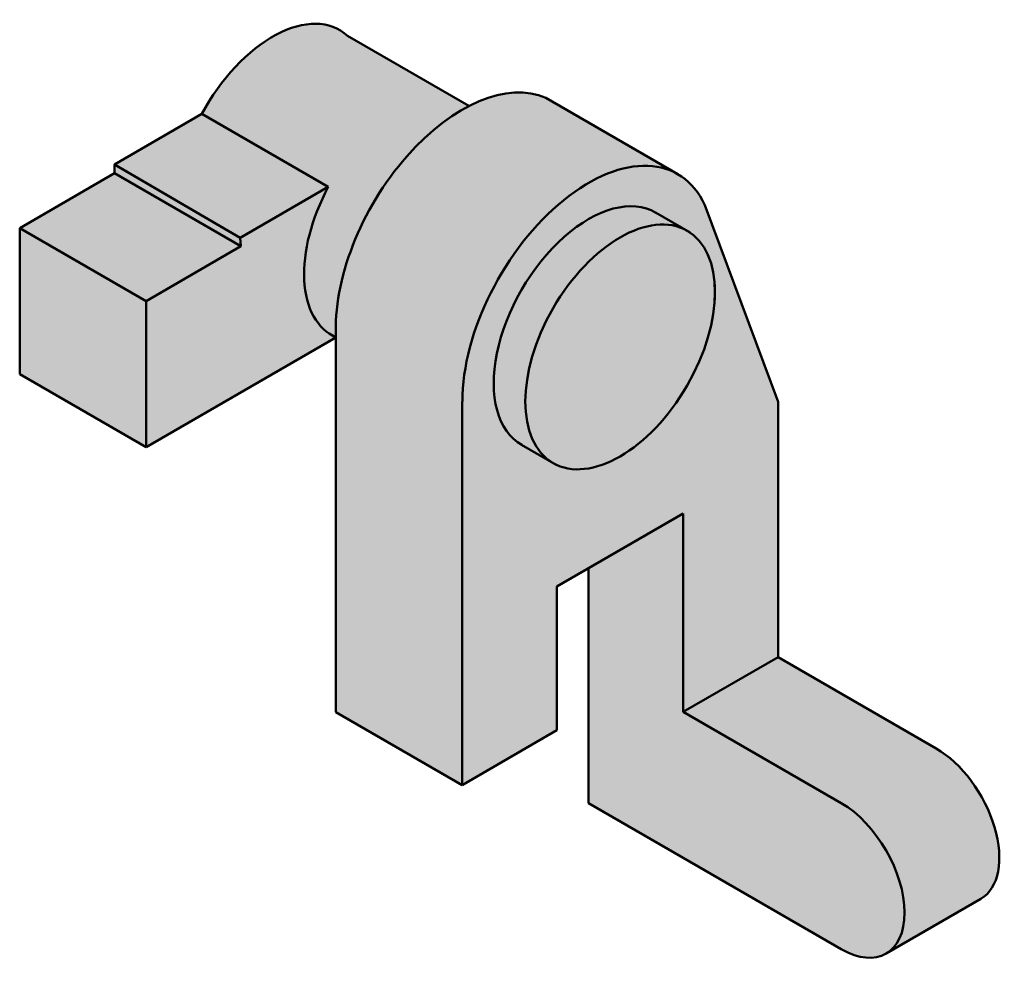
# Model space of a CAD drawing. Units: millimetres. Extents: x -330 to -195, y 135 to 265.
import ezdxf

# ---------------------------------------------------------------- set-up
doc = ezdxf.new("R2010")
doc.units = ezdxf.units.MM
doc.header["$MEASUREMENT"] = 0
doc.layers.add('M-HATC', color=18, linetype='Continuous', lineweight=18)
doc.layers.add('M-OUTL', color=18, linetype='Continuous', lineweight=50)

msp = doc.modelspace()

# ---------------------------------------------------------------- hatches: boundary and pattern name
at = {"layer": 'M-HATC'}
h = msp.add_hatch(color=256, dxfattribs=at)
h.dxf.hatch_style = 1
h.set_gradient(color1=(205, 105, 40), color2=(254, 234, 185), tint=1)
edge = h.paths.add_edge_path()
edge.add_line((-239.4440334627808, 243.7158516808131), (-257.507454304211, 254.1447725660983))
edge.add_ellipse((-268.9894374735072, 232.5417108040857), major_axis=(-12.24744871391589, -21.21320343559643), ratio=0.577350269189626, start_angle=182.0094469365693, end_angle=207.4091084575104)
edge.add_ellipse((-268.9894374735072, 232.5417108040857), major_axis=(-12.24744871391589, -21.21320343559643), ratio=0.577350269189626, start_angle=207.4091084575104, end_angle=332.9239439551128)
edge.add_line((-286.2780511034371, 221.3469536046194), (-286.2780511034371, 170.0048822703966))
edge.add_line((-286.2780511034371, 170.0048822703966), (-268.9894374735072, 160.0232965372411))
edge.add_line((-268.9894374735072, 160.0232965372411), (-255.9990564167406, 167.5232965372411))
edge.add_line((-255.9990564167406, 167.5232965372411), (-255.9990564167406, 187.2014834929562))
edge.add_line((-255.9990564167406, 187.2014834929562), (-238.6785483410518, 197.2014834929561))
edge.add_line((-238.6785483410518, 197.2014834929561), (-238.6785483410518, 170.0417108040857))
edge.add_line((-238.6785483410518, 170.0417108040857), (-225.6881672842852, 177.5417108040857))
edge.add_line((-225.6881672842852, 177.5417108040857), (-225.6881672842852, 212.5048822703966))
edge.add_line((-225.6881672842852, 212.5048822703966), (-235.7183808055639, 239.4515141482783))
edge.add_ellipse((-251.6689293978184, 222.5417108040857), major_axis=(-12.22489593503758, -21.17414087672732), ratio=0.577350269189626, start_angle=166.6720954430869, end_angle=180)
edge = h.paths.add_edge_path(flags=16)
edge.add_ellipse((-251.6689293978184, 222.5417108040857), major_axis=(-9.18558653543692, -15.90990257669731), ratio=0.5773502691896257, start_angle=179.9999999999978, end_angle=360.0000000000009, ccw=False)
edge.add_ellipse((-251.6689293978184, 222.5417108040857), major_axis=(-9.18558653543692, -15.90990257669731), ratio=0.5773502691896257, start_angle=179.8699372542578, end_angle=179.9999999999978, ccw=False)
edge.add_line((-242.4472982318591, 238.4306390373698), (-238.5387202913605, 236.1562404709099))
edge.add_ellipse((-247.3388023788962, 220.0417108040857), major_axis=(-9.18558653543692, -15.90990257669731), ratio=0.5773502691896257, start_angle=178.5085589172631, end_angle=181.3612175018271, ccw=False)
edge.add_ellipse((-247.3388023788962, 220.0417108040857), major_axis=(-9.18558653543692, -15.90990257669731), ratio=0.5773502691896257, start_angle=153.3615057074265, end_angle=178.5085589172631, ccw=False)
edge.add_ellipse((-247.3388023788962, 220.0417108040857), major_axis=(-9.18558653543692, -15.90990257669731), ratio=0.5773502691896257, start_angle=146.3945410341213, end_angle=153.3615057074265, ccw=False)
edge.add_ellipse((-247.3388023788962, 220.0417108040857), major_axis=(-9.18558653543692, -15.90990257669731), ratio=0.5773502691896257, start_angle=1.4914410827216216, end_angle=146.3945410341213, ccw=False)
edge.add_ellipse((-247.3388023788962, 220.0417108040857), major_axis=(-9.18558653543692, -15.90990257669731), ratio=0.5773502691896257, start_angle=358.6387824981857, end_angle=361.4914410827216, ccw=False)
edge.add_line((-256.894353396639, 204.363351327481), (-260.8183293037713, 206.6110798333951))
edge.add_ellipse((-251.6689293978184, 222.5417108040857), major_axis=(-9.18558653543692, -15.90990257669731), ratio=0.5773502691896257, start_angle=360.0000000000009, end_angle=360.130062745741, ccw=False)
edge = h.paths.add_edge_path()
edge.add_ellipse((-204.0375321896743, 155.0417108040857), major_axis=(6.123724356957941, -10.60660171779822), ratio=0.577350269189626, start_angle=0, end_angle=150)
edge.add_line((-204.0375321896743, 165.0417108040857), (-225.6881672842852, 177.5417108040857))
edge.add_line((-225.6881672842852, 177.5417108040857), (-238.6785483410518, 170.0417108040857))
edge.add_line((-238.6785483410518, 170.0417108040857), (-217.0279132464409, 157.5417108040857))
edge.add_ellipse((-217.0279132464409, 147.5417108040857), major_axis=(6.123724356957941, -10.60660171779822), ratio=0.577350269189626, start_angle=359.99999999999994, end_angle=510, ccw=False)
edge.add_line((-210.904188889483, 136.9351090862874), (-197.9138078327163, 144.4351090862875))
edge = h.paths.add_edge_path()
edge.add_ellipse((-217.0279132464409, 147.5417108040857), major_axis=(6.123724356957941, -10.60660171779822), ratio=0.577350269189626, start_angle=360, end_angle=510)
edge.add_line((-217.0279132464411, 157.5417108040859), (-238.6785483410518, 170.0417108040857))
edge.add_line((-238.6785483410518, 170.0417108040857), (-238.6785483410518, 197.2014834929561))
edge.add_line((-238.6785483410518, 197.2014834929561), (-251.6689293978184, 189.7014834929562))
edge.add_line((-251.6689293978184, 189.7014834929562), (-251.6689293978184, 157.5417108040857))
edge.add_line((-251.6689293978184, 157.5417108040857), (-238.6785483410518, 150.0417108040857))
edge.add_line((-238.6785483410518, 150.0417108040857), (-217.0279132464409, 137.5417108040857))
edge.add_ellipse((-217.0279132464409, 147.5417108040857), major_axis=(6.123724356957941, -10.60660171779822), ratio=0.577350269189626, start_angle=330.0000000000001, end_angle=360)
edge = h.paths.add_edge_path()
edge.add_ellipse((-277.6496915113515, 237.5417108040857), major_axis=(-9.18558653543692, -15.90990257669731), ratio=0.5773502691896257, start_angle=275.5133311571051, end_angle=361.95187951225597, ccw=False)
edge.add_line((-287.3321498768701, 241.9515408603362), (-299.3853540072795, 234.9926202110469))
edge.add_line((-299.3853540072795, 234.9926202110469), (-299.3003266059625, 233.8285393377748))
edge.add_line((-299.3003266059625, 233.8285393377748), (-312.2907076627291, 226.3285393377748))
edge.add_line((-312.2907076627291, 226.3285393377748), (-312.2907076627291, 206.3285393377748))
edge.add_line((-312.2907076627291, 206.3285393377748), (-286.2780511034371, 221.3469536046194))
edge = h.paths.add_edge_path()
edge.add_ellipse((-268.9894374735072, 232.5417108040857), major_axis=(-12.24744871391589, -21.21320343559643), ratio=0.577350269189626, start_angle=207.4091084575104, end_angle=332.92394395511286, ccw=False)
edge.add_line((-268.0614854647615, 253.048740355375), (-284.6964083784061, 262.6529175775164))
edge.add_ellipse((-294.9701995870403, 247.5417108040857), major_axis=(-9.18558653543692, -15.90990257669731), ratio=0.5773502691896257, start_angle=175.789041267969, end_angle=275.5133311571049)
edge.add_line((-304.6526579525588, 251.9515408603362), (-316.6208346816513, 245.0417108040857))
edge.add_line((-316.6208346816513, 245.0417108040857), (-299.3853540072795, 234.9926202110469))
edge.add_line((-299.3853540072795, 234.9926202110469), (-287.3321498768701, 241.9515408603362))
edge.add_ellipse((-277.6496915113515, 237.5417108040857), major_axis=(-9.18558653543692, -15.90990257669731), ratio=0.5773502691896257, start_angle=275.513331157105, end_angle=361.951879512256)
h.paths.add_polyline_path([(-316.6208346816513, 243.8285393377748), (-329.6112157384179, 236.3285393377748), (-312.2907076627291, 226.3285393377748), (-299.3003266059625, 233.8285393377748)])
h.paths.add_polyline_path([(-312.2907076627291, 226.3285393377748), (-329.6112157384178, 236.3285393377748), (-329.6112157384179, 216.3285393377748), (-312.2907076627291, 206.3285393377748)])
edge = h.paths.add_edge_path(flags=0)
edge.add_ellipse((-247.3388023788962, 220.0417108040857), major_axis=(-9.18558653543692, -15.90990257669731), ratio=0.5773502691896257, start_angle=1.491441082721595, end_angle=146.3945410341212)
edge.add_line((-234.3803157678885, 226.4728206118725), (-234.3803157678885, 228.5737724626098))
edge.add_ellipse((-247.3388023788962, 220.0417108040857), major_axis=(-9.18558653543692, -15.90990257669731), ratio=0.5773502691896257, start_angle=153.3615057074265, end_angle=178.5085589172631)
edge.add_line((-237.748725305762, 235.6965429824348), (-238.5387202913641, 236.1562404709116))
edge.add_ellipse((-247.3388023788962, 220.0417108040857), major_axis=(-9.18558653543692, -15.90990257669731), ratio=0.5773502691896257, start_angle=181.3612175018105, end_angle=358.6387824981857)
edge.add_line((-256.894353396639, 204.363351327481), (-256.1012462007659, 203.9090443453283))
edge = h.paths.add_edge_path(flags=0)
edge.add_ellipse((-247.3388023788962, 220.0417108040857), major_axis=(-9.18558653543692, -15.90990257669731), ratio=0.5773502691896257, start_angle=181.3612175018106, end_angle=358.6387824981857, ccw=False)
edge.add_line((-238.5387202913624, 236.1562404709111), (-242.4833428623707, 238.4516133807787))
edge.add_ellipse((-251.6689293978184, 222.5417108040857), major_axis=(-9.18558653543692, -15.90990257669731), ratio=0.5773502691896257, start_angle=179.9999999999978, end_angle=360.0000000000009)
edge.add_line((-260.8545159332551, 206.6318082273883), (-256.894353396639, 204.3633513274811))
h = msp.add_hatch(color=256, dxfattribs=at)
h.dxf.hatch_style = 1
h.set_gradient(color1=(205, 105, 40), color2=(254, 234, 185), tint=1)
edge = h.paths.add_edge_path()
edge.add_ellipse((-247.3388023788962, 220.0417108040857), major_axis=(-9.18558653543692, -15.90990257669731), ratio=0.5773502691896257, start_angle=1.491441082721595, end_angle=146.3945410341212)
edge.add_line((-234.3803157678885, 226.4728206118725), (-234.3803157678885, 228.5737724626099))
edge.add_ellipse((-247.3388023788962, 220.0417108040857), major_axis=(-9.18558653543692, -15.90990257669731), ratio=0.5773502691896257, start_angle=153.3615057074265, end_angle=178.5085589172631)
edge.add_line((-237.748725305762, 235.6965429824348), (-238.5387202913671, 236.1562404709133))
edge.add_ellipse((-247.3388023788962, 220.0417108040857), major_axis=(-9.18558653543692, -15.90990257669731), ratio=0.5773502691896257, start_angle=181.361217501827, end_angle=358.6387824981857)
edge.add_line((-256.894353396639, 204.3633513274811), (-256.1012462007659, 203.9090443453283))
edge = h.paths.add_edge_path()
edge.add_ellipse((-247.3388023788962, 220.0417108040857), major_axis=(-9.18558653543692, -15.90990257669731), ratio=0.5773502691896257, start_angle=181.3612175018271, end_angle=358.6387824981857, ccw=False)
edge.add_line((-238.5387202913672, 236.1562404709133), (-242.4833428623809, 238.4516133807827))
edge.add_ellipse((-251.6689293978184, 222.5417108040857), major_axis=(-9.18558653543692, -15.90990257669731), ratio=0.5773502691896257, start_angle=179.9999999999978, end_angle=360.0000000000009)
edge.add_line((-260.8545159332551, 206.6318082273883), (-256.894353396639, 204.3633513274811))
h.paths.add_polyline_path([(-316.6208346816513, 245.0417108040857), (-316.6208346816513, 243.8285393377748), (-299.3003266059625, 233.8285393377748), (-299.3853540072795, 234.9926202110469)])

# ---------------------------------------------------------------- linework, layer by layer
at = {"layer": 'M-OUTL'}
for p, q in [((-284.696408378406, 262.6529175775163), (-268.0614854647615, 253.048740355375)), ((-239.4440334627808, 243.7158516808131), (-257.507454304211, 254.1447725660983)), ((-304.6526579525588, 251.9515408603362), (-316.6208346816513, 245.0417108040857)), ((-287.3319348696171, 241.9518300562505), (-304.6524429453059, 251.9518300562505)), ((-316.6208346816513, 243.8285393377748), (-316.6208346816513, 245.0417108040857)), ((-316.6208346816513, 245.0417108040857), (-299.3853540072795, 234.9926202110469)), ((-329.6112157384178, 236.3285393377748), (-316.6208346816513, 243.8285393377748)), ((-299.3003266059625, 233.8285393377748), (-316.6208346816513, 243.8285393377748)), ((-299.3853540072795, 234.9926202110469), (-287.3321498768701, 241.9515408603362)), ((-225.6881672842852, 212.5048822703966), (-235.7183808055629, 239.4515141482755)), ((-242.4833428623815, 238.451613380783), (-237.748725305762, 235.6965429824348)), ((-329.6112157384178, 236.3285393377748), (-329.6112157384178, 216.3285393377748)), ((-312.2907076627291, 226.3285393377748), (-329.6112157384178, 236.3285393377748)), ((-299.3003266059625, 233.8285393377748), (-299.3853540072795, 234.9926202110469)), ((-312.2907076627291, 226.3285393377748), (-299.3003266059625, 233.8285393377748)), ((-234.3803157678885, 228.5737724626098), (-234.3803157678885, 226.4728206118725)), ((-312.2907076627291, 226.3285393377748), (-312.2907076627291, 206.3285393377748)), ((-312.2907076627291, 206.3285393377748), (-312.2907076627291, 226.3285393377748)), ((-286.2780511034371, 221.3469536046194), (-312.2907076627291, 206.3285393377748)), ((-286.2780511034371, 221.3469536046194), (-286.2780511034371, 170.0048822703966)), ((-312.2907076627291, 206.3285393377748), (-329.6112157384178, 216.3285393377748)), ((-268.9894374735072, 212.5417108040857), (-268.9894374735072, 160.0232965372411)), ((-225.6881672842852, 212.5048822703966), (-225.6881672842852, 177.5417108040857)), ((-260.8545159332553, 206.6318082273884), (-256.1012462007659, 203.9090443453283)), ((-238.6785483410518, 197.2014834929561), (-255.9990564167406, 187.2014834929562)), ((-238.6785483410518, 170.0417108040857), (-238.6785483410518, 197.2014834929561)), ((-251.6689293978184, 189.7014834929562), (-251.6689293978184, 157.5417108040857)), ((-268.9894374735072, 160.0232965372411), (-268.9894374735072, 187.5048822703966)), ((-255.9990564167406, 167.5232965372411), (-255.9990564167406, 187.2014834929562)), ((-238.6785483410518, 170.0417108040857), (-225.6881672842852, 177.5417108040857)), ((-204.0375321896743, 165.0417108040857), (-225.6881672842852, 177.5417108040857)), ((-268.9894374735072, 160.0232965372411), (-286.2780511034371, 170.0048822703966)), ((-217.0279132464409, 157.5417108040857), (-238.6785483410518, 170.0417108040857)), ((-268.9894374735072, 160.0232965372411), (-255.9990564167406, 167.5232965372411)), ((-238.6785483410518, 150.0417108040857), (-251.6689293978184, 157.5417108040857)), ((-238.6785483410518, 150.0417108040857), (-217.0279132464409, 137.5417108040857)), ((-210.9041888894829, 136.9351090862875), (-197.9138078327163, 144.4351090862875))]:
    msp.add_line(p, q, dxfattribs=at)
for centre, major_axis, ratio, start_param, end_param in [((-294.9701995870403, 247.5417108040857), (-9.18558653543692, -15.90990257669731), 0.5773502691896257, 3.014750379593766, 4.768059487555172), ((-268.9894374735072, 232.5417108040857), (-12.24744871391589, -21.21320343559643), 0.577350269189626, 3.202288487123413, 5.558482977315758), ((-277.2831166307185, 237.1598121220914), (-9.18558653543692, -15.90990257669731), 0.5773502691896257, 3.137660871671104, 3.145524435508498), ((-251.6689293978184, 222.5417108040857), (-12.22489593503758, -21.17414087672732), 0.577350269189626, 2.752212726052509, 5.497787143782137), ((-277.6496915113515, 237.5417108040857), (-9.18558653543692, -15.90990257669731), 0.5773502691896257, 4.768059487555174, 6.342145026113557), ((-251.6689293978184, 222.5417108040857), (-9.18558653543692, -15.90990257669731), 0.5773502691896257, 3.137660871671104, 6.287117089098234), ((-204.0375321896743, 155.0417108040857), (6.123724356957941, -10.60660171779822), 0.5773502691896262, 0, 2.356194490192345), ((-217.0279132464409, 147.5417108040857), (6.123724356957941, -10.60660171779822), 0.5773502691896262, 5.497787143782138, 8.63937979737193)]:
    msp.add_ellipse(centre, major_axis=major_axis, ratio=ratio, start_param=start_param, end_param=end_param, dxfattribs=at)
msp.add_ellipse((-247.3388023788962, 220.0417108040857), major_axis=(-9.18558653543692, -15.90990257669731), ratio=0.5773502691896257, dxfattribs=at)

doc.saveas('drawing.dxf')
